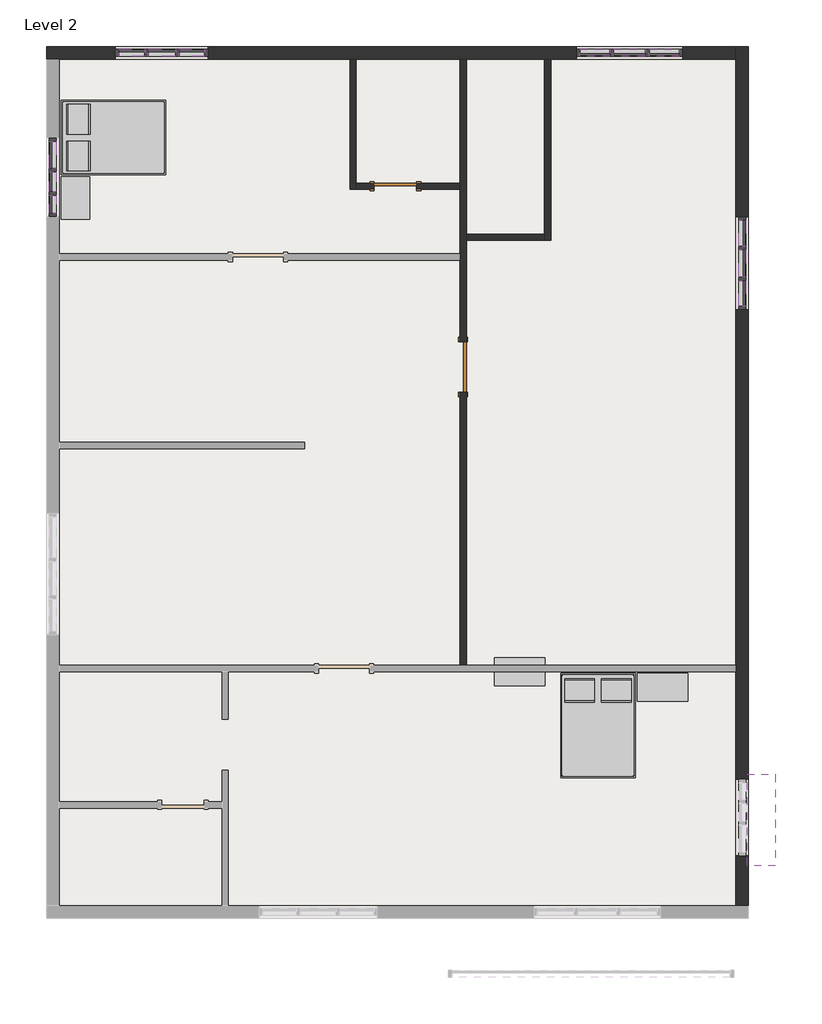
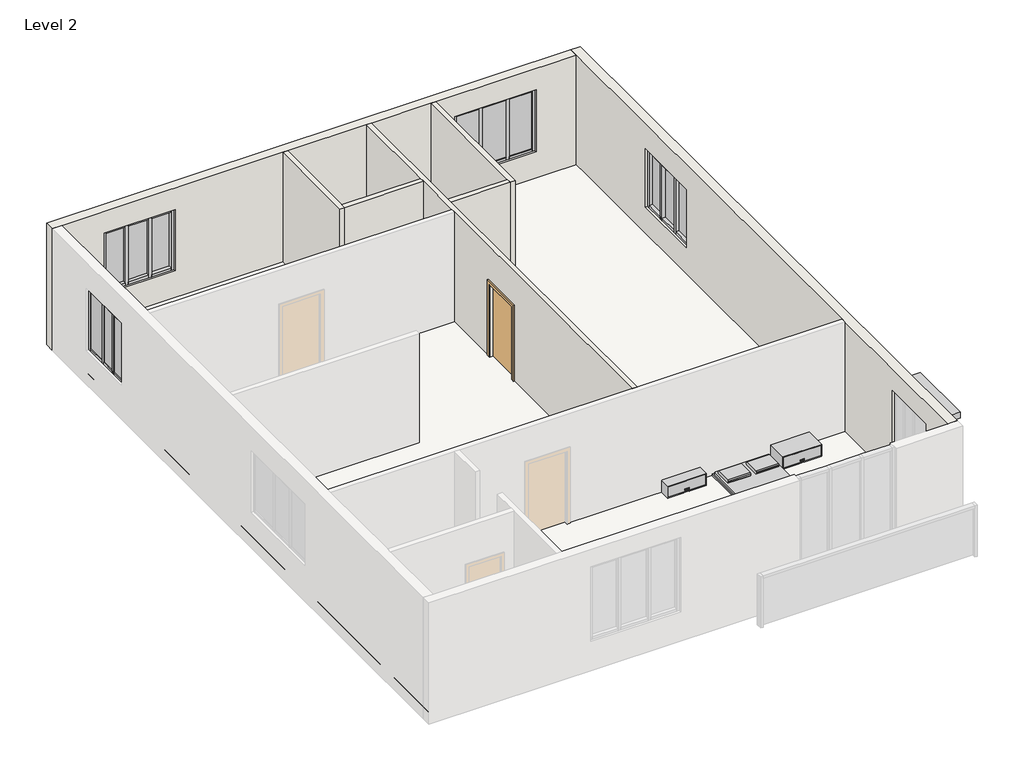
# One storey, part 2 of 2: 40 members, 12 plates, 7 walls, 5 furniture elements, 2 doors, 1 proxy, 1 roof.
"""IFC4 building model written with IfcOpenShell, lengths in millimetres."""

from ifc_helpers import new_model, si_unit, frame, origin, place, context, project, spatial, polyline, outline, extrude, faceted_brep, transform, mapped, element, save
from components import generic_models_5_generic_models_5_415a3505, door_f2b275c1, door_e5f9f3c4, furniture_b58f7881, furniture_6b884072, furniture_fb07e05e, member_a980948f, member_2ebf4a73, member_5535eeb3, member_b9f3750b, member_e606cc0e, member_d09add03, member_f2991489, member_1ff484d5, member_830eb86c, member_2edf994d, member_fb9f8cdf, member_2891061c, member_06776a95, member_f05129a9, member_20042e51, system_panel_glazed_3f13655f, system_panel_glazed_13fbf6b0, system_panel_glazed_7c06924b, system_panel_glazed_6a435647, system_panel_glazed_74412268, system_panel_glazed_37901f3f, system_panel_glazed_2ffdee7e, system_panel_glazed_b9e07fbe, system_panel_glazed_76557058

model = new_model("IFC4")

# Units and contexts
model_context = context("Model", 3, world=origin())
ifc_project = project(units=[si_unit("LENGTHUNIT", "METRE", prefix="MILLI")], contexts=[model_context])

# Site, building, storey
site = spatial("IfcSite", under=ifc_project)
building = spatial("IfcBuilding", under=site)
storey = spatial("IfcBuildingStorey", under=building, Name="Level 2", Elevation=3048.0)

# Proxy
placement = place(None, origin())
generic_models_5_generic_models_5_shape = generic_models_5_generic_models_5_415a3505(model_context)
element("IfcBuildingElementProxy", 1, Name="Generic Models 5 : Generic Models 5", ObjectType="Generic Models 5 : Generic Models 5", at=placement, inside=storey, context=model_context, shape_type="MappedRepresentation", body=[
    mapped(generic_models_5_generic_models_5_shape, transform((0.0, 0.0, 0.0), x_axis=(1.0, 0.0, 0.0), y_axis=(0.0, 1.0, 0.0), z_axis=(0.0, 0.0, 1.0))),
])

# Doors
door_shape = door_f2b275c1(model_context)
element("IfcDoor", 2, ObjectType="Single-Flush : 30\" x 80\"", at=placement, inside=storey, context=model_context, shape_type="MappedRepresentation", body=[
    mapped(door_shape, transform((-17179.0386697, 977.9488046, 3048.0), x_axis=(-1.0, 0.0, 0.0), y_axis=(0.0, -1.0, 0.0), z_axis=(0.0, 0.0, 1.0))),
])
door_2_shape = door_e5f9f3c4(model_context)
element("IfcDoor", 3, ObjectType="Single-Flush : 36\" x 84\"", at=placement, inside=storey, context=model_context, shape_type="MappedRepresentation", body=[
    mapped(door_2_shape, transform((-15959.8386697, -2279.6011954, 3048.0), x_axis=(0.0, -1.0, 0.0), y_axis=(1.0, 0.0, 0.0), z_axis=(0.0, 0.0, 1.0))),
])

# Furniture
furniture_shape = furniture_b58f7881(model_context)
element("IfcFurniture", 4, ObjectType="Bed-Box : Double 53\" x 74\"", at=placement, inside=storey, context=model_context, shape_type="MappedRepresentation", body=[
    mapped(furniture_shape, transform((-13866.9411288, -8498.2643194, 3048.0), x_axis=(1.0, 0.0, 0.0), y_axis=(0.0, 1.0, 0.0), z_axis=(0.0, 0.0, 1.0))),
])
element("IfcFurniture", 5, ObjectType="Bed-Box : Double 53\" x 74\"", at=placement, inside=storey, context=model_context, shape_type="MappedRepresentation", body=[
    mapped(furniture_shape, transform((-22493.4681779, 1515.0963456, 3048.0), x_axis=(0.0, 1.0, 0.0), y_axis=(-1.0, 0.0, 0.0), z_axis=(0.0, 0.0, 1.0))),
])
furniture_2_shape = furniture_6b884072(model_context)
element("IfcFurniture", 6, ObjectType="Cabinet File-Lateral 2 Drawer : 36\" x 20\" x 24\"", at=placement, inside=storey, context=model_context, shape_type="MappedRepresentation", body=[
    mapped(furniture_2_shape, transform((-12185.7161558, -7112.5754515, 3048.0), x_axis=(1.0, 0.0, 0.0), y_axis=(0.0, 1.0, 0.0), z_axis=(0.0, 0.0, 1.0))),
])
element("IfcFurniture", 7, ObjectType="Cabinet File-Lateral 2 Drawer : 36\" x 20\" x 24\"", at=placement, inside=storey, context=model_context, shape_type="MappedRepresentation", body=[
    mapped(furniture_2_shape, transform((-14757.4661558, -6831.6828193, 3048.0), x_axis=(1.0, 0.0, 0.0), y_axis=(0.0, 1.0, 0.0), z_axis=(0.0, 0.0, 1.0))),
])
furniture_3_shape = furniture_fb07e05e(model_context)
element("IfcFurniture", 8, ObjectType="Cabinet File-Lateral 3 Drawer : 30\" x 20\" x 36\"", at=placement, inside=storey, context=model_context, shape_type="MappedRepresentation", body=[
    mapped(furniture_3_shape, transform((-23879.1570458, 944.6737776, 3048.0), x_axis=(0.0, 1.0, 0.0), y_axis=(-1.0, 0.0, 0.0), z_axis=(0.0, 0.0, 1.0))),
])

# Members
member_shape = member_a980948f(model_context)
element("IfcMember", 9, ObjectType="Rectangular Mullion : 2.5\" x 5\" rectangular", at=placement, inside=storey, context=model_context, shape_type="MappedRepresentation", body=[
    mapped(member_shape, transform((-12607.0386697, 3378.2488046, 5569.0204449), x_axis=(0.0, 0.0, 1.0), y_axis=(0.0, 1.0, 0.0), z_axis=(-1.0, 0.0, 0.0))),
])
element("IfcMember", 10, ObjectType="Rectangular Mullion : 2.5\" x 5\" rectangular", at=placement, inside=storey, context=model_context, shape_type="MappedRepresentation", body=[
    mapped(member_shape, transform((-13857.9886697, 3378.2488046, 5569.0204449), x_axis=(0.0, 0.0, 1.0), y_axis=(0.0, 1.0, 0.0), z_axis=(-1.0, 0.0, 0.0))),
])
element("IfcMember", 11, ObjectType="Rectangular Mullion : 2.5\" x 5\" rectangular", at=placement, inside=storey, context=model_context, shape_type="MappedRepresentation", body=[
    mapped(member_shape, transform((-13311.8886697, 3378.2488046, 4006.889054), x_axis=(0.0, 0.0, -1.0), y_axis=(0.0, 1.0, 0.0), z_axis=(1.0, 0.0, 0.0))),
])
element("IfcMember", 12, ObjectType="Rectangular Mullion : 2.5\" x 5\" rectangular", at=placement, inside=storey, context=model_context, shape_type="MappedRepresentation", body=[
    mapped(member_shape, transform((-12060.9386697, 3378.2488046, 4006.889054), x_axis=(0.0, 0.0, -1.0), y_axis=(0.0, 1.0, 0.0), z_axis=(1.0, 0.0, 0.0))),
])
member_2_shape = member_2ebf4a73(model_context)
element("IfcMember", 13, ObjectType="Rectangular Mullion : 2.5\" x 5\" rectangular", at=placement, inside=storey, context=model_context, shape_type="MappedRepresentation", body=[
    mapped(member_2_shape, transform((-10930.6386697, -660.3511954, 5470.7760363), x_axis=(0.0, 0.0, 1.0), y_axis=(-1.0, 0.0, 0.0), z_axis=(0.0, -1.0, 0.0))),
])
element("IfcMember", 14, ObjectType="Rectangular Mullion : 2.5\" x 5\" rectangular", at=placement, inside=storey, context=model_context, shape_type="MappedRepresentation", body=[
    mapped(member_2_shape, transform((-21141.4386697, 3378.2488046, 5548.8556249), x_axis=(0.0, 0.0, 1.0), y_axis=(0.0, -1.0, 0.0), z_axis=(1.0, 0.0, 0.0))),
])
member_3_shape = member_5535eeb3(model_context)
element("IfcMember", 15, ObjectType="Rectangular Mullion : 2.5\" x 5\" rectangular", at=placement, inside=storey, context=model_context, shape_type="MappedRepresentation", body=[
    mapped(member_3_shape, transform((-10930.6386697, -101.5511954, 5470.7760363), x_axis=(0.0, 0.0, 1.0), y_axis=(-1.0, 0.0, 0.0), z_axis=(0.0, -1.0, 0.0))),
])
element("IfcMember", 16, ObjectType="Rectangular Mullion : 2.5\" x 5\" rectangular", at=placement, inside=storey, context=model_context, shape_type="MappedRepresentation", body=[
    mapped(member_3_shape, transform((-10930.6386697, -1187.4011954, 5470.7760363), x_axis=(0.0, 0.0, 1.0), y_axis=(-1.0, 0.0, 0.0), z_axis=(0.0, -1.0, 0.0))),
])
element("IfcMember", 17, ObjectType="Rectangular Mullion : 2.5\" x 5\" rectangular", at=placement, inside=storey, context=model_context, shape_type="MappedRepresentation", body=[
    mapped(member_3_shape, transform((-21700.2386697, 3378.2488046, 5548.8556249), x_axis=(0.0, 0.0, 1.0), y_axis=(0.0, -1.0, 0.0), z_axis=(1.0, 0.0, 0.0))),
])
element("IfcMember", 18, ObjectType="Rectangular Mullion : 2.5\" x 5\" rectangular", at=placement, inside=storey, context=model_context, shape_type="MappedRepresentation", body=[
    mapped(member_3_shape, transform((-20614.3886697, 3378.2488046, 5548.8556249), x_axis=(0.0, 0.0, 1.0), y_axis=(0.0, -1.0, 0.0), z_axis=(1.0, 0.0, 0.0))),
])
element("IfcMember", 19, ObjectType="Rectangular Mullion : 2.5\" x 5\" rectangular", at=placement, inside=storey, context=model_context, shape_type="MappedRepresentation", body=[
    mapped(member_3_shape, transform((-10930.6386697, -723.8511954, 4008.2774218), x_axis=(0.0, 0.0, -1.0), y_axis=(-1.0, 0.0, 0.0), z_axis=(0.0, 1.0, 0.0))),
])
element("IfcMember", 20, ObjectType="Rectangular Mullion : 2.5\" x 5\" rectangular", at=placement, inside=storey, context=model_context, shape_type="MappedRepresentation", body=[
    mapped(member_3_shape, transform((-10930.6386697, 361.9988046, 4008.2774218), x_axis=(0.0, 0.0, -1.0), y_axis=(-1.0, 0.0, 0.0), z_axis=(0.0, 1.0, 0.0))),
])
element("IfcMember", 21, ObjectType="Rectangular Mullion : 2.5\" x 5\" rectangular", at=placement, inside=storey, context=model_context, shape_type="MappedRepresentation", body=[
    mapped(member_3_shape, transform((-21077.9386697, 3378.2488046, 4019.4962213), x_axis=(0.0, 0.0, -1.0), y_axis=(0.0, -1.0, 0.0), z_axis=(-1.0, 0.0, 0.0))),
])
element("IfcMember", 22, ObjectType="Rectangular Mullion : 2.5\" x 5\" rectangular", at=placement, inside=storey, context=model_context, shape_type="MappedRepresentation", body=[
    mapped(member_3_shape, transform((-22163.7886697, 3378.2488046, 4019.4962213), x_axis=(0.0, 0.0, -1.0), y_axis=(0.0, -1.0, 0.0), z_axis=(-1.0, 0.0, 0.0))),
])
element("IfcMember", 23, ObjectType="Rectangular Mullion : 2.5\" x 5\" rectangular", at=placement, inside=storey, context=model_context, shape_type="MappedRepresentation", body=[
    mapped(member_2_shape, transform((-10930.6386697, -165.0511954, 4008.2774218), x_axis=(0.0, 0.0, -1.0), y_axis=(-1.0, 0.0, 0.0), z_axis=(0.0, 1.0, 0.0))),
])
element("IfcMember", 24, ObjectType="Rectangular Mullion : 2.5\" x 5\" rectangular", at=placement, inside=storey, context=model_context, shape_type="MappedRepresentation", body=[
    mapped(member_2_shape, transform((-21636.7386697, 3378.2488046, 4019.4962213), x_axis=(0.0, 0.0, -1.0), y_axis=(0.0, -1.0, 0.0), z_axis=(-1.0, 0.0, 0.0))),
])
member_4_shape = member_b9f3750b(model_context)
element("IfcMember", 25, ObjectType="Rectangular Mullion : 2.5\" x 5\" rectangular", at=placement, inside=storey, context=model_context, shape_type="MappedRepresentation", body=[
    mapped(member_4_shape, transform((-23351.2386697, 1790.7488046, 5453.2250414), x_axis=(0.0, 0.0, 1.0), y_axis=(1.0, 0.0, 0.0), z_axis=(0.0, 1.0, 0.0))),
])
element("IfcMember", 26, ObjectType="Rectangular Mullion : 2.5\" x 5\" rectangular", at=placement, inside=storey, context=model_context, shape_type="MappedRepresentation", body=[
    mapped(member_4_shape, transform((-23351.2386697, 1301.7988046, 3896.5069058), x_axis=(0.0, 0.0, -1.0), y_axis=(1.0, 0.0, 0.0), z_axis=(0.0, -1.0, 0.0))),
])
member_5_shape = member_e606cc0e(model_context)
element("IfcMember", 27, ObjectType="Rectangular Mullion : 2.5\" x 5\" rectangular", at=placement, inside=storey, context=model_context, shape_type="MappedRepresentation", body=[
    mapped(member_5_shape, transform((-10930.6386697, -692.1011954, 4008.2774218), x_axis=(0.0, -1.0, 0.0), y_axis=(-1.0, 0.0, 0.0), z_axis=(0.0, 0.0, -1.0))),
])
element("IfcMember", 28, ObjectType="Rectangular Mullion : 2.5\" x 5\" rectangular", at=placement, inside=storey, context=model_context, shape_type="MappedRepresentation", body=[
    mapped(member_5_shape, transform((-10930.6386697, -133.3011954, 4008.2774218), x_axis=(0.0, -1.0, 0.0), y_axis=(-1.0, 0.0, 0.0), z_axis=(0.0, 0.0, -1.0))),
])
member_6_shape = member_d09add03(model_context)
element("IfcMember", 29, ObjectType="Rectangular Mullion : 2.5\" x 5\" rectangular", at=placement, inside=storey, context=model_context, shape_type="MappedRepresentation", body=[
    mapped(member_6_shape, transform((-10930.6386697, -1250.9011954, 4008.2774218), x_axis=(0.0, -1.0, 0.0), y_axis=(-1.0, 0.0, 0.0), z_axis=(0.0, 0.0, -1.0))),
])
element("IfcMember", 30, ObjectType="Rectangular Mullion : 2.5\" x 5\" rectangular", at=placement, inside=storey, context=model_context, shape_type="MappedRepresentation", body=[
    mapped(member_6_shape, transform((-10930.6386697, 425.4988046, 5470.7760363), x_axis=(0.0, 1.0, 0.0), y_axis=(-1.0, 0.0, 0.0), z_axis=(0.0, 0.0, 1.0))),
])
member_7_shape = member_f2991489(model_context)
element("IfcMember", 31, ObjectType="Rectangular Mullion : 2.5\" x 5\" rectangular", at=placement, inside=storey, context=model_context, shape_type="MappedRepresentation", body=[
    mapped(member_7_shape, transform((-21109.6886697, 3378.2488046, 4019.4962213), x_axis=(1.0, 0.0, 0.0), y_axis=(0.0, -1.0, 0.0), z_axis=(0.0, 0.0, -1.0))),
])
element("IfcMember", 32, ObjectType="Rectangular Mullion : 2.5\" x 5\" rectangular", at=placement, inside=storey, context=model_context, shape_type="MappedRepresentation", body=[
    mapped(member_7_shape, transform((-21668.4886697, 3378.2488046, 4019.4962213), x_axis=(1.0, 0.0, 0.0), y_axis=(0.0, -1.0, 0.0), z_axis=(0.0, 0.0, -1.0))),
])
member_8_shape = member_1ff484d5(model_context)
element("IfcMember", 33, ObjectType="Rectangular Mullion : 2.5\" x 5\" rectangular", at=placement, inside=storey, context=model_context, shape_type="MappedRepresentation", body=[
    mapped(member_8_shape, transform((-20550.8886697, 3378.2488046, 4019.4962213), x_axis=(1.0, 0.0, 0.0), y_axis=(0.0, -1.0, 0.0), z_axis=(0.0, 0.0, -1.0))),
])
element("IfcMember", 34, ObjectType="Rectangular Mullion : 2.5\" x 5\" rectangular", at=placement, inside=storey, context=model_context, shape_type="MappedRepresentation", body=[
    mapped(member_8_shape, transform((-22227.2886697, 3378.2488046, 5548.8556249), x_axis=(-1.0, 0.0, 0.0), y_axis=(0.0, -1.0, 0.0), z_axis=(0.0, 0.0, 1.0))),
])
member_9_shape = member_830eb86c(model_context)
element("IfcMember", 35, ObjectType="Rectangular Mullion : 2.5\" x 5\" rectangular", at=placement, inside=storey, context=model_context, shape_type="MappedRepresentation", body=[
    mapped(member_9_shape, transform((-13248.3886697, 3378.2488046, 5569.0204449), x_axis=(0.0, 0.0, 1.0), y_axis=(0.0, 1.0, 0.0), z_axis=(-1.0, 0.0, 0.0))),
])
member_10_shape = member_2edf994d(model_context)
element("IfcMember", 36, ObjectType="Rectangular Mullion : 2.5\" x 5\" rectangular", at=placement, inside=storey, context=model_context, shape_type="MappedRepresentation", body=[
    mapped(member_10_shape, transform((-12638.7886697, 3378.2488046, 4006.889054), x_axis=(-1.0, 0.0, 0.0), y_axis=(0.0, 1.0, 0.0), z_axis=(0.0, 0.0, -1.0))),
])
element("IfcMember", 37, ObjectType="Rectangular Mullion : 2.5\" x 5\" rectangular", at=placement, inside=storey, context=model_context, shape_type="MappedRepresentation", body=[
    mapped(member_10_shape, transform((-13280.1386697, 3378.2488046, 4006.889054), x_axis=(-1.0, 0.0, 0.0), y_axis=(0.0, 1.0, 0.0), z_axis=(0.0, 0.0, -1.0))),
])
element("IfcMember", 38, ObjectType="Rectangular Mullion : 2.5\" x 5\" rectangular", at=placement, inside=storey, context=model_context, shape_type="MappedRepresentation", body=[
    mapped(member_9_shape, transform((-12670.5386697, 3378.2488046, 4006.889054), x_axis=(0.0, 0.0, -1.0), y_axis=(0.0, 1.0, 0.0), z_axis=(1.0, 0.0, 0.0))),
])
member_11_shape = member_fb9f8cdf(model_context)
element("IfcMember", 39, ObjectType="Rectangular Mullion : 2.5\" x 5\" rectangular", at=placement, inside=storey, context=model_context, shape_type="MappedRepresentation", body=[
    mapped(member_11_shape, transform((-11997.4386697, 3378.2488046, 5569.0204449), x_axis=(1.0, 0.0, 0.0), y_axis=(0.0, 1.0, 0.0), z_axis=(0.0, 0.0, 1.0))),
])
element("IfcMember", 40, ObjectType="Rectangular Mullion : 2.5\" x 5\" rectangular", at=placement, inside=storey, context=model_context, shape_type="MappedRepresentation", body=[
    mapped(member_11_shape, transform((-13921.4886697, 3378.2488046, 4006.889054), x_axis=(-1.0, 0.0, 0.0), y_axis=(0.0, 1.0, 0.0), z_axis=(0.0, 0.0, -1.0))),
])
member_12_shape = member_2891061c(model_context)
element("IfcMember", 41, ObjectType="Rectangular Mullion : 2.5\" x 5\" rectangular", at=placement, inside=storey, context=model_context, shape_type="MappedRepresentation", body=[
    mapped(member_12_shape, transform((-23351.2386697, 816.0238046, 5453.2250414), x_axis=(0.0, 0.0, 1.0), y_axis=(1.0, 0.0, 0.0), z_axis=(0.0, 1.0, 0.0))),
])
member_13_shape = member_06776a95(model_context)
element("IfcMember", 42, ObjectType="Rectangular Mullion : 2.5\" x 5\" rectangular", at=placement, inside=storey, context=model_context, shape_type="MappedRepresentation", body=[
    mapped(member_13_shape, transform((-23351.2386697, 1238.2988046, 5453.2250414), x_axis=(0.0, 0.0, 1.0), y_axis=(1.0, 0.0, 0.0), z_axis=(0.0, 1.0, 0.0))),
])
member_14_shape = member_f05129a9(model_context)
element("IfcMember", 43, ObjectType="Rectangular Mullion : 2.5\" x 5\" rectangular", at=placement, inside=storey, context=model_context, shape_type="MappedRepresentation", body=[
    mapped(member_14_shape, transform((-23351.2386697, 1270.0488046, 3896.5069058), x_axis=(0.0, 1.0, 0.0), y_axis=(1.0, 0.0, 0.0), z_axis=(0.0, 0.0, -1.0))),
])
element("IfcMember", 44, ObjectType="Rectangular Mullion : 2.5\" x 5\" rectangular", at=placement, inside=storey, context=model_context, shape_type="MappedRepresentation", body=[
    mapped(member_14_shape, transform((-23351.2386697, 847.7738046, 3896.5069058), x_axis=(0.0, 1.0, 0.0), y_axis=(1.0, 0.0, 0.0), z_axis=(0.0, 0.0, -1.0))),
])
element("IfcMember", 45, ObjectType="Rectangular Mullion : 2.5\" x 5\" rectangular", at=placement, inside=storey, context=model_context, shape_type="MappedRepresentation", body=[
    mapped(member_13_shape, transform((-23351.2386697, 879.5238046, 3896.5069058), x_axis=(0.0, 0.0, -1.0), y_axis=(1.0, 0.0, 0.0), z_axis=(0.0, -1.0, 0.0))),
])
element("IfcMember", 46, ObjectType="Rectangular Mullion : 2.5\" x 5\" rectangular", at=placement, inside=storey, context=model_context, shape_type="MappedRepresentation", body=[
    mapped(member_12_shape, transform((-23351.2386697, 488.9988046, 3896.5069058), x_axis=(0.0, 0.0, -1.0), y_axis=(1.0, 0.0, 0.0), z_axis=(0.0, -1.0, 0.0))),
])
member_15_shape = member_20042e51(model_context)
element("IfcMember", 47, ObjectType="Rectangular Mullion : 2.5\" x 5\" rectangular", at=placement, inside=storey, context=model_context, shape_type="MappedRepresentation", body=[
    mapped(member_15_shape, transform((-23351.2386697, 425.4988046, 5453.2250414), x_axis=(0.0, -1.0, 0.0), y_axis=(1.0, 0.0, 0.0), z_axis=(0.0, 0.0, 1.0))),
])
element("IfcMember", 48, ObjectType="Rectangular Mullion : 2.5\" x 5\" rectangular", at=placement, inside=storey, context=model_context, shape_type="MappedRepresentation", body=[
    mapped(member_15_shape, transform((-23351.2386697, 1854.2488046, 3896.5069058), x_axis=(0.0, 1.0, 0.0), y_axis=(1.0, 0.0, 0.0), z_axis=(0.0, 0.0, -1.0))),
])

# Plates
system_panel_glazed_shape = system_panel_glazed_3f13655f(model_context)
element("IfcPlate", 49, ObjectType="System Panel : Glazed", at=placement, inside=storey, context=model_context, shape_type="MappedRepresentation", body=[
    mapped(system_panel_glazed_shape, transform((-10930.6386697, 130.2238046, 4071.7774218), x_axis=(0.0, -1.0, 0.0), y_axis=(1.0, 0.0, 0.0), z_axis=(0.0, 0.0, 1.0))),
])
element("IfcPlate", 50, ObjectType="System Panel : Glazed", at=placement, inside=storey, context=model_context, shape_type="MappedRepresentation", body=[
    mapped(system_panel_glazed_shape, transform((-10930.6386697, -955.6261954, 4071.7774218), x_axis=(0.0, -1.0, 0.0), y_axis=(1.0, 0.0, 0.0), z_axis=(0.0, 0.0, 1.0))),
])
system_panel_glazed_2_shape = system_panel_glazed_13fbf6b0(model_context)
element("IfcPlate", 51, ObjectType="System Panel : Glazed", at=placement, inside=storey, context=model_context, shape_type="MappedRepresentation", body=[
    mapped(system_panel_glazed_2_shape, transform((-10930.6386697, -412.7011954, 4071.7774218), x_axis=(0.0, -1.0, 0.0), y_axis=(1.0, 0.0, 0.0), z_axis=(0.0, 0.0, 1.0))),
])
system_panel_glazed_3_shape = system_panel_glazed_7c06924b(model_context)
element("IfcPlate", 52, ObjectType="System Panel : Glazed", at=placement, inside=storey, context=model_context, shape_type="MappedRepresentation", body=[
    mapped(system_panel_glazed_3_shape, transform((-21932.0136697, 3378.2488046, 4082.9962213), x_axis=(1.0, 0.0, 0.0), y_axis=(0.0, 1.0, 0.0), z_axis=(0.0, 0.0, 1.0))),
])
element("IfcPlate", 53, ObjectType="System Panel : Glazed", at=placement, inside=storey, context=model_context, shape_type="MappedRepresentation", body=[
    mapped(system_panel_glazed_3_shape, transform((-20846.1636697, 3378.2488046, 4082.9962213), x_axis=(1.0, 0.0, 0.0), y_axis=(0.0, 1.0, 0.0), z_axis=(0.0, 0.0, 1.0))),
])
system_panel_glazed_4_shape = system_panel_glazed_6a435647(model_context)
element("IfcPlate", 54, ObjectType="System Panel : Glazed", at=placement, inside=storey, context=model_context, shape_type="MappedRepresentation", body=[
    mapped(system_panel_glazed_4_shape, transform((-21389.0886697, 3378.2488046, 4082.9962213), x_axis=(1.0, 0.0, 0.0), y_axis=(0.0, 1.0, 0.0), z_axis=(0.0, 0.0, 1.0))),
])
system_panel_glazed_5_shape = system_panel_glazed_74412268(model_context)
element("IfcPlate", 55, ObjectType="System Panel : Glazed", at=placement, inside=storey, context=model_context, shape_type="MappedRepresentation", body=[
    mapped(system_panel_glazed_5_shape, transform((-12333.9886697, 3378.2488046, 4070.389054), x_axis=(-1.0, 0.0, 0.0), y_axis=(0.0, -1.0, 0.0), z_axis=(0.0, 0.0, 1.0))),
])
element("IfcPlate", 56, ObjectType="System Panel : Glazed", at=placement, inside=storey, context=model_context, shape_type="MappedRepresentation", body=[
    mapped(system_panel_glazed_5_shape, transform((-13584.9386697, 3378.2488046, 4070.389054), x_axis=(-1.0, 0.0, 0.0), y_axis=(0.0, -1.0, 0.0), z_axis=(0.0, 0.0, 1.0))),
])
system_panel_glazed_6_shape = system_panel_glazed_37901f3f(model_context)
element("IfcPlate", 57, ObjectType="System Panel : Glazed", at=placement, inside=storey, context=model_context, shape_type="MappedRepresentation", body=[
    mapped(system_panel_glazed_6_shape, transform((-12959.4636697, 3378.2488046, 4070.389054), x_axis=(-1.0, 0.0, 0.0), y_axis=(0.0, -1.0, 0.0), z_axis=(0.0, 0.0, 1.0))),
])
system_panel_glazed_7_shape = system_panel_glazed_2ffdee7e(model_context)
element("IfcPlate", 58, ObjectType="System Panel : Glazed", at=placement, inside=storey, context=model_context, shape_type="MappedRepresentation", body=[
    mapped(system_panel_glazed_7_shape, transform((-23351.2386697, 652.5113046, 3960.0069058), x_axis=(0.0, 1.0, 0.0), y_axis=(-1.0, 0.0, 0.0), z_axis=(0.0, 0.0, 1.0))),
])
system_panel_glazed_8_shape = system_panel_glazed_b9e07fbe(model_context)
element("IfcPlate", 59, ObjectType="System Panel : Glazed", at=placement, inside=storey, context=model_context, shape_type="MappedRepresentation", body=[
    mapped(system_panel_glazed_8_shape, transform((-23351.2386697, 1546.2738046, 3960.0069058), x_axis=(0.0, 1.0, 0.0), y_axis=(-1.0, 0.0, 0.0), z_axis=(0.0, 0.0, 1.0))),
])
system_panel_glazed_9_shape = system_panel_glazed_76557058(model_context)
element("IfcPlate", 60, ObjectType="System Panel : Glazed", at=placement, inside=storey, context=model_context, shape_type="MappedRepresentation", body=[
    mapped(system_panel_glazed_9_shape, transform((-23351.2386697, 1058.9113046, 3960.0069058), x_axis=(0.0, 1.0, 0.0), y_axis=(-1.0, 0.0, 0.0), z_axis=(0.0, 0.0, 1.0))),
])

# Roof
element("IfcRoof", 61, ObjectType="Generic - 12\"", at=placement, inside=storey, context=model_context, shape_type="SweptSolid", body=[
    extrude(outline(polyline([(-23465.5386697, 3492.5488046), (-10816.3386697, 3492.5488046), (-10816.3386697, -12204.6511954), (-23465.5386697, -12204.6511954), (-23465.5386697, 3492.5488046)])), frame((0.0, 0.0, 3048.0), z_axis=(0.0, 0.0, 1.0), x_axis=(1.0, 0.0, 0.0)), (0.0, 0.0, 1.0), 304.8),
])

# Walls
element("IfcWall", 62, ObjectType="4.5\"", at=placement, inside=storey, context=model_context, shape_type="Brep", body=[
    faceted_brep([(-16016.9886697, -2736.8011954, 5181.6), (-16016.9886697, -2736.8011954, 3048.0), (-16016.9886697, -7651.7011954, 3048.0), (-16016.9886697, -7651.7011954, 6096.0), (-16016.9886697, -355.5511954, 6096.0), (-16016.9886697, -241.2511954, 6096.0), (-16016.9886697, 920.7988046, 6096.0), (-16016.9886697, 1035.0988046, 6096.0), (-16016.9886697, 3263.9488046, 6096.0), (-16016.9886697, 3263.9488046, 3048.0), (-16016.9886697, 1035.0988046, 3048.0), (-16016.9886697, 920.7988046, 3048.0), (-16016.9886697, -241.2511954, 3048.0), (-16016.9886697, -355.5511954, 3048.0), (-16016.9886697, -1822.4011954, 3048.0), (-16016.9886697, -1822.4011954, 5181.6), (-15902.6886697, -7651.7011954, 3048.0), (-15902.6886697, -2736.8011954, 3048.0), (-15902.6886697, -2736.8011954, 5181.6), (-15902.6886697, -1822.4011954, 5181.6), (-15902.6886697, -1822.4011954, 3048.0), (-15902.6886697, 0.0488046, 3048.0), (-15902.6886697, 114.3488046, 3048.0), (-15902.6886697, 3263.9488046, 3048.0), (-15902.6886697, 3263.9488046, 6096.0), (-15902.6886697, 114.3488046, 6096.0), (-15902.6886697, 0.0488046, 6096.0), (-15902.6886697, -7651.7011954, 6096.0)], [[[0, 1, 2, 3, 4, 5, 6, 7, 8, 9, 10, 11, 12, 13, 14, 15]], [[16, 17, 18, 19, 20, 21, 22, 23, 24, 25, 26, 27]], [[2, 1, 17, 16]], [[14, 13, 12, 11, 10, 9, 23, 22, 21, 20]], [[8, 7, 6, 5, 4, 3, 27, 26, 25, 24]], [[9, 8, 24, 23]], [[3, 2, 16, 27]], [[18, 17, 1, 0]], [[19, 18, 0, 15]], [[20, 19, 15, 14]]]),
])
element("IfcWall", 63, ObjectType="4.5\"", at=placement, inside=storey, context=model_context, shape_type="Brep", body=[
    faceted_brep([(-14378.6886697, 0.0488046, 3048.0), (-14378.6886697, 3263.9488046, 3048.0), (-14378.6886697, 3263.9488046, 6096.0), (-14378.6886697, 0.0488046, 6096.0), (-14492.9886697, 0.0488046, 3048.0), (-14492.9886697, 0.0488046, 6096.0), (-14492.9886697, 114.3488046, 6096.0), (-14492.9886697, 3263.9488046, 6096.0), (-14492.9886697, 3263.9488046, 3048.0), (-14492.9886697, 114.3488046, 3048.0)], [[[0, 1, 2, 3]], [[4, 5, 6, 7, 8, 9]], [[1, 0, 4, 9, 8]], [[3, 2, 7, 6, 5]], [[2, 1, 8, 7]], [[0, 3, 5, 4]]]),
])
element("IfcWall", 64, ObjectType="4.5\"", at=placement, inside=storey, context=model_context, shape_type="Brep", body=[
    faceted_brep([(-17998.1886697, 3263.9488046, 3048.0), (-17998.1886697, 920.7988046, 3048.0), (-17998.1886697, 920.7988046, 6096.0), (-17998.1886697, 3263.9488046, 6096.0), (-17883.8886697, 3263.9488046, 3048.0), (-17883.8886697, 3263.9488046, 6096.0), (-17883.8886697, 1035.0988046, 6096.0), (-17883.8886697, 920.7988046, 6096.0), (-17883.8886697, 920.7988046, 3048.0), (-17883.8886697, 1035.0988046, 3048.0)], [[[0, 1, 2, 3]], [[4, 5, 6, 7, 8, 9]], [[1, 0, 4, 9, 8]], [[3, 2, 7, 6, 5]], [[0, 3, 5, 4]], [[2, 1, 8, 7]]]),
])
element("IfcWall", 65, ObjectType="4.5\"", at=placement, inside=storey, context=model_context, shape_type="SweptSolid", body=[
    extrude(outline(polyline([(3048.0, -17883.8886697), (3048.0, -17560.0386697), (5080.0, -17560.0386697), (5080.0, -16798.0386697), (3048.0, -16798.0386697), (3048.0, -16016.9886697), (6096.0, -16016.9886697), (6096.0, -17883.8886697), (3048.0, -17883.8886697)])), frame((0.0, 920.7988046, 0.0), z_axis=(0.0, 1.0, 0.0), x_axis=(0.0, 0.0, 1.0)), (0.0, 0.0, 1.0), 114.3),
])
element("IfcWall", 66, ObjectType="4.5\"", at=placement, inside=storey, context=model_context, shape_type="SweptSolid", body=[
    extrude(outline(polyline([(-15902.6886697, 114.3488046), (-14492.9886697, 114.3488046), (-14492.9886697, 0.0488046), (-15902.6886697, 0.0488046), (-15902.6886697, 114.3488046)])), frame((0.0, 0.0, 3048.0), z_axis=(0.0, 0.0, 1.0), x_axis=(1.0, 0.0, 0.0)), (0.0, 0.0, 1.0), 3048.0),
])
element("IfcWall", 67, ObjectType="9\"", at=placement, inside=storey, context=model_context, shape_type="Brep", body=[
    faceted_brep([(-10816.3386697, -11976.0511954, 3048.0), (-10816.3386697, 3492.5488046, 3048.0), (-10816.3386697, 3492.5488046, 6096.0), (-10816.3386697, -11976.0511954, 6096.0), (-10816.3386697, -11077.5261954, 4038.9192224), (-10816.3386697, -11077.5261954, 5551.780974), (-10816.3386697, -9705.9261954, 5551.780974), (-10816.3386697, -9705.9261954, 4038.9192224), (-10816.3386697, 425.4988046, 5470.7760363), (-10816.3386697, 425.4988046, 4008.2774218), (-10816.3386697, -1250.9011954, 4008.2774218), (-10816.3386697, -1250.9011954, 5470.7760363), (-11044.9386697, 3492.5488046, 3048.0), (-11044.9386697, 3263.9488046, 3048.0), (-11044.9386697, -7651.7011954, 3048.0), (-11044.9386697, -7766.0011954, 3048.0), (-11044.9386697, -11976.0511954, 3048.0), (-11044.9386697, -11976.0511954, 6096.0), (-11044.9386697, -7766.0011954, 6096.0), (-11044.9386697, -7651.7011954, 6096.0), (-11044.9386697, 3263.9488046, 6096.0), (-11044.9386697, 3492.5488046, 6096.0), (-11044.9386697, -11077.5261954, 5551.780974), (-11044.9386697, -11077.5261954, 4038.9192224), (-11044.9386697, -9705.9261954, 4038.9192224), (-11044.9386697, -9705.9261954, 5551.780974), (-11044.9386697, 425.4988046, 4008.2774218), (-11044.9386697, 425.4988046, 5470.7760363), (-11044.9386697, -1250.9011954, 5470.7760363), (-11044.9386697, -1250.9011954, 4008.2774218)], [[[0, 1, 2, 3], [4, 5, 6, 7], [8, 9, 10, 11]], [[12, 13, 14, 15, 16, 17, 18, 19, 20, 21], [22, 23, 24, 25], [26, 27, 28, 29]], [[1, 0, 16, 15, 14, 13, 12]], [[3, 2, 21, 20, 19, 18, 17]], [[0, 3, 17, 16]], [[2, 1, 12, 21]], [[22, 5, 4, 23]], [[5, 22, 25, 6]], [[6, 25, 24, 7]], [[23, 4, 7, 24]], [[26, 9, 8, 27]], [[27, 8, 11, 28]], [[28, 11, 10, 29]], [[9, 26, 29, 10]]]),
])
element("IfcWall", 68, ObjectType="9\"", at=placement, inside=storey, context=model_context, shape_type="Brep", body=[
    faceted_brep([(-11044.9386697, 3492.5488046, 3048.0), (-23465.5386697, 3492.5488046, 3048.0), (-23465.5386697, 3492.5488046, 6096.0), (-11044.9386697, 3492.5488046, 6096.0), (-22227.2886697, 3492.5488046, 5548.8556249), (-22227.2886697, 3492.5488046, 4019.4962213), (-20550.8886697, 3492.5488046, 4019.4962213), (-20550.8886697, 3492.5488046, 5548.8556249), (-11997.4386697, 3492.5488046, 4006.889054), (-11997.4386697, 3492.5488046, 5569.0204449), (-13921.4886697, 3492.5488046, 5569.0204449), (-13921.4886697, 3492.5488046, 4006.889054), (-23465.5386697, 3263.9488046, 3048.0), (-23236.9386697, 3263.9488046, 3048.0), (-17998.1886697, 3263.9488046, 3048.0), (-17883.8886697, 3263.9488046, 3048.0), (-16016.9886697, 3263.9488046, 3048.0), (-15902.6886697, 3263.9488046, 3048.0), (-14492.9886697, 3263.9488046, 3048.0), (-14378.6886697, 3263.9488046, 3048.0), (-11044.9386697, 3263.9488046, 3048.0), (-11044.9386697, 3263.9488046, 6096.0), (-14378.6886697, 3263.9488046, 6096.0), (-14492.9886697, 3263.9488046, 6096.0), (-15902.6886697, 3263.9488046, 6096.0), (-16016.9886697, 3263.9488046, 6096.0), (-17883.8886697, 3263.9488046, 6096.0), (-17998.1886697, 3263.9488046, 6096.0), (-23236.9386697, 3263.9488046, 6096.0), (-23465.5386697, 3263.9488046, 6096.0), (-22227.2886697, 3263.9488046, 4019.4962213), (-22227.2886697, 3263.9488046, 5548.8556249), (-20550.8886697, 3263.9488046, 5548.8556249), (-20550.8886697, 3263.9488046, 4019.4962213), (-11997.4386697, 3263.9488046, 5569.0204449), (-11997.4386697, 3263.9488046, 4006.889054), (-13921.4886697, 3263.9488046, 4006.889054), (-13921.4886697, 3263.9488046, 5569.0204449)], [[[0, 1, 2, 3], [4, 5, 6, 7], [8, 9, 10, 11]], [[12, 13, 14, 15, 16, 17, 18, 19, 20, 21, 22, 23, 24, 25, 26, 27, 28, 29], [30, 31, 32, 33], [34, 35, 36, 37]], [[1, 0, 20, 19, 18, 17, 16, 15, 14, 13, 12]], [[3, 2, 29, 28, 27, 26, 25, 24, 23, 22, 21]], [[0, 3, 21, 20]], [[2, 1, 12, 29]], [[4, 31, 30, 5]], [[31, 4, 7, 32]], [[32, 7, 6, 33]], [[5, 30, 33, 6]], [[8, 35, 34, 9]], [[9, 34, 37, 10]], [[10, 37, 36, 11]], [[35, 8, 11, 36]]]),
])

save(model, "model.ifc")

# Revit data of these elements
# Type "Single-Flush : 30\" x 80\""
#   Type Mark = "5"
#   Construction Type Id = "MDOOR"
#   Assembly Code = "C1020"
#   Analytic Construction = "Metal"
#   Thickness = 0' - 2"
#   Heat Transfer Coefficient (U) = 0.651978 BTU/(h·ft²·°F)
#   Height = 6' - 8"
#   Trim Projection Ext = 0' - 1"
#   Trim Projection Int = 0' - 1"
#   Trim Width = 0' - 3"
#   Width = 2' - 6"
#   Define Thermal Properties by = 1
#   Define Thermal Properties by = 1
#   Door Material = Door - Panel
#   Frame Material = Door - Frame
#   Visual Light Transmittance = 0
#   Solar Heat Gain Coefficient = 0
#   Function = (empty or 0)
#   Wall Closure = (empty or 0)
# Type "Single-Flush : 36\" x 84\""
#   Type Mark = "1"
#   Construction Type Id = "MDOOR"
#   Assembly Code = "C1020"
#   Analytic Construction = "Metal"
#   Thickness = 0' - 2"
#   Heat Transfer Coefficient (U) = 0.651978 BTU/(h·ft²·°F)
#   Height = 7' - 0"
#   Trim Projection Ext = 0' - 1"
#   Trim Projection Int = 0' - 1"
#   Trim Width = 0' - 3"
#   Width = 3' - 0"
#   Define Thermal Properties by = 1
#   Define Thermal Properties by = 1
#   Door Material = Door - Panel
#   Frame Material = Door - Frame
#   Visual Light Transmittance = 0
#   Solar Heat Gain Coefficient = 0
#   Function = (empty or 0)
#   Wall Closure = (empty or 0)
# Type "Bed-Box : Double 53\" x 74\""
#   Assembly Code = "E2020200"
#   Length = 6' - 2"
#   Width = 4' - 5"
#   Frame Material = Birch
#   Mattress Material = Linen, White
#   Default Elevation = 0
# Type "Cabinet File-Lateral 2 Drawer : 36\" x 20\" x 24\""
#   Assembly Code = "E2020200"
#   Depth = 1' - 8"
#   Height = 2' - 0"
#   Width = 3' - 0"
#   Material = Metal - Steel
#   Default Elevation = 0
# Type "Cabinet File-Lateral 3 Drawer : 30\" x 20\" x 36\""
#   Assembly Code = "E2020200"
#   Depth = 1' - 8"
#   Height = 3' - 0"
#   Width = 2' - 6"
#   Material = Metal - Steel
#   Default Elevation = 0
# Type "Rectangular Mullion : 2.5\" x 5\" rectangular"
#   built-in parameter 1007304 = 0.416667 (stored number, unit not read)
#   built-in parameter 1007301 = 0.104167 (stored number, unit not read)
#   built-in parameter 1007300 = 0.104167 (stored number, unit not read)
# Type "System Panel : Glazed"
#   Construction Type Id = "GSP4R"
#   Analytic Construction = "1/8 in Pilkington single glazing"
#   Visual Light Transmittance = 0.9
#   Solar Heat Gain Coefficient = 0.86
#   Heat Transfer Coefficient (U) = 1.18115 BTU/(h·ft²·°F)
#   Define Thermal Properties by = 1
# Type "Generic - 12\""
#   Assembly Code = "B1020"
#   Layers, outside or top first: 1' - 0" no material (function 1)
# Type "4.5\""
#   Assembly Code = "B2010"
#   Layers, outside or top first: 0' - 4 1/2" no material (function 1)
# Type "9\""
#   Assembly Code = "B2010"
#   Layers, outside or top first: 0' - 9" no material (function 1)
# Element 1 (IfcBuildingElementProxy, "Generic Models 5 : Generic Models 5")
#   Phase Created = New Construction
# Element 2 (IfcDoor, "Single-Flush : 30\" x 80\"")
#   Phase Created = New Construction
#   Materials on its faces: "Door - Frame", "Door - Panel"
# Element 3 (IfcDoor, "Single-Flush : 36\" x 84\"")
#   Phase Created = New Construction
#   Materials on its faces: "Door - Frame", "Door - Panel"
# Elements 4, 5 (IfcFurniture, "Bed-Box : Double 53\" x 74\"")
#   Phase Created = New Construction
#   Materials on its faces: "Birch", "Linen, White"
# Elements 6, 7 (IfcFurniture, "Cabinet File-Lateral 2 Drawer : 36\" x 20\" x 24\"")
#   Phase Created = New Construction
#   Materials on its faces: "Metal - Steel"
# Element 8 (IfcFurniture, "Cabinet File-Lateral 3 Drawer : 30\" x 20\" x 36\"")
#   Phase Created = New Construction
#   Materials on its faces: "Metal - Steel"
# Elements 9, 10, 11, 12, 13, 14, 15, 16, 17, 18, 19, 20, 21, 22, 23, 24, 25, 26, 27, 28, 29, 30, 31, 32, 33, 34, 35, 36, 37, 38, 39, 40, 41, 42, 43, 44, 45, 46, 47, 48 (IfcMember, "Rectangular Mullion : 2.5\" x 5\" rectangular")
#   Phase Created = New Construction
#   Materials on its faces: "Aluminum"
# Elements 49, 50, 51, 52, 53, 54, 55, 56, 57, 58, 59, 60 (IfcPlate, "System Panel : Glazed")
#   Phase Created = New Construction
#   Materials on its faces: "Glass"
# Element 61 (IfcRoof, "Generic - 12\"")
#   built-in parameter 1001705 = 11 (stored number, unit not read)
#   built-in parameter 1001710 = 33615
#   Phase Created = New Construction
#   Materials on its faces: "Default Roof"
# Elements 62, 63, 64, 65, 66 (IfcWall, "4.5\"")
#   Top Offset = 0' - 0"
#   Base Offset = 0' - 0"
#   Unconnected Height = 10' - 0"
#   wall height = 10' - 0"
#   Phase Created = New Construction
#   Base Constraint = Level 2
#   Materials on its faces: "Default Wall"
# Elements 67, 68 (IfcWall, "9\"")
#   Top Offset = 0' - 0"
#   Base Offset = 0' - 0"
#   Unconnected Height = 10' - 0"
#   wall height = 10' - 0"
#   Phase Created = New Construction
#   Base Constraint = Level 2
#   Materials on its faces: "Default Wall"
# Materials
#   "Door - Panel": class "Wood", colour RGB 210 159 95, transparency 0, Cost = 0
#   "Door - Frame": colour RGB 118 70 51, transparency 0, Cost = 0
#   "Birch": class "Wood", colour RGB 224 178 126, transparency 0, Description = "Betula Alleghaniensis", Cost = 0
#   "Linen, White": class "Textile", colour RGB 247 247 239, transparency 0, Description = "Linen, white", Cost = 0
#   "Metal - Steel": colour RGB 209 209 209, transparency 0
#   "Aluminum": class "Metal", colour RGB 247 247 247, transparency 0, Description = "Aluminum 6061", Cost = 0
#   "Glass": class "Glass", colour RGB 0 128 192, transparency 0.75, Description = "Soda Lime Glass", Cost = 0
#   "Default Roof": colour RGB 88 101 114, transparency 0, Cost = 0
#   "Default Wall": colour RGB 128 128 128, transparency 0, Cost = 0
